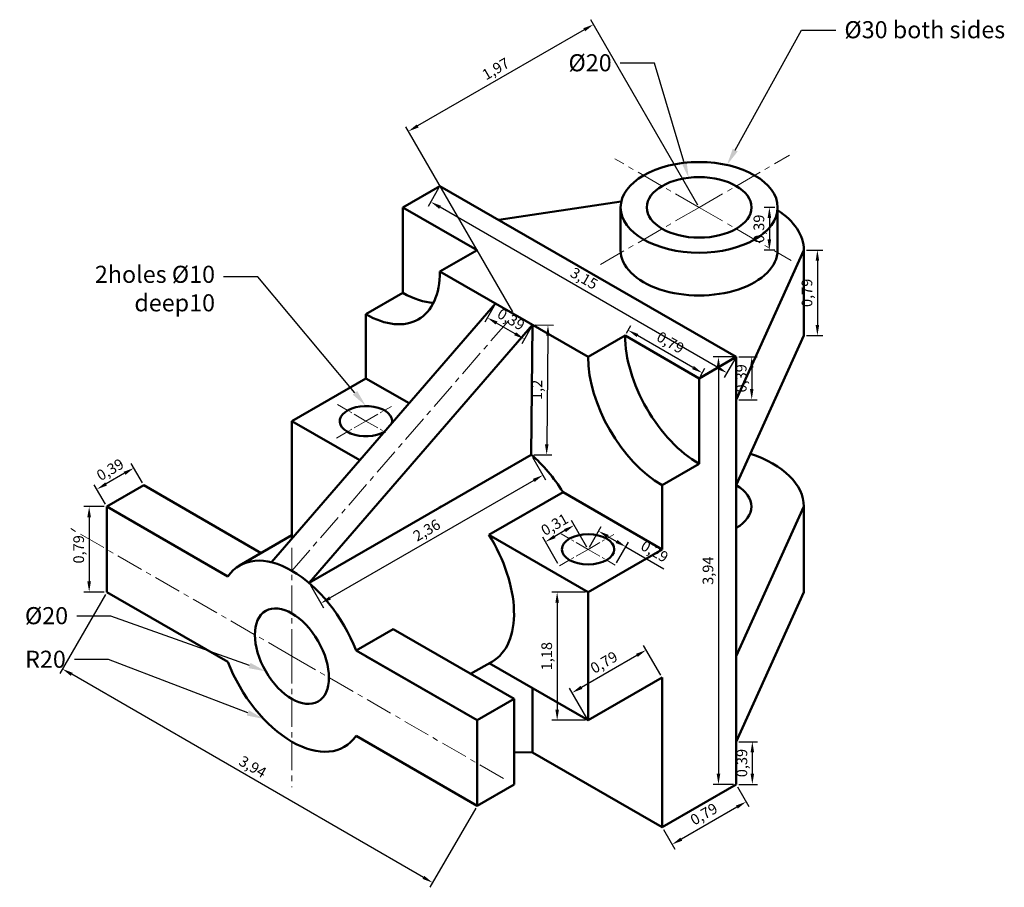
# Model space of a CAD drawing. Units: inches. Extents: x 1453 to 39065, y 1991 to 51453.
# Tile 1 of 1: x 1452.7 to 1683, y 1990.8 to 2193.8. Entities that reach past the tile are written whole.
import ezdxf
from ezdxf import colors
from ezdxf.entities.mleader import LeaderData, LeaderLine
from ezdxf.math import Vec2, Vec3

# ---------------------------------------------------------------- set-up
doc = ezdxf.new("R2010")
doc.units = ezdxf.units.IN
doc.linetypes.add('CENTER', pattern=[50.8, 31.75, -6.35, 6.35, -6.35])
for name, color, linetype, lineweight in [('M-CNTR', 1, 'CENTER', 18), ('M-DIMS', 2, 'Continuous', 25), ('M-OUTL', 7, 'Continuous', 50), ('M-TEXT', 3, 'Continuous', 25)]:
    doc.layers.add(name, color=color, linetype=linetype, lineweight=lineweight)
doc.styles.get("Standard").update_dxf_attribs({"font": 'arial.ttf'})
doc.dimstyles.new('ISO-25', dxfattribs={"dimtxt": 2.5, "dimasz": 2.5, "dimexe": 1.25, "dimexo": 0.625, "dimtad": 1, "dimtxsty": 'Standard', "dimcen": 2.5, "dimadec": 0, "dimazin": 0, "dimtfac": 1, "dimtmove": 0, "dimatfit": 3, "dimfxl": 1, "dimarcsym": 0})

# ---------------------------------------------------------------- blocks, each defined once
blk = doc.blocks.new('*D1')
at = {"layer": 'Defpoints', "color": 0, "transparency": 16777216}
for p in [(1563.98, 2127.35), (1562.07, 2124.04), (1572.64, 2122.35)]:
    blk.add_point(p, dxfattribs=at)
at = {"layer": 'M-DIMS', "color": 0, "lineweight": -2, "transparency": 16777216}
for p, q in [((1563.67, 2126.81), (1561.45, 2122.96)), ((1568.57, 2120.29), (1564.24, 2122.79)), ((1572.33, 2121.81), (1570.11, 2117.96))]:
    blk.add_line(p, q, dxfattribs=at)
at = {"layer": 'M-DIMS', "color": 0, "transparency": 16777216}
for points in [[(1564.45, 2123.15), (1564.03, 2122.43), (1562.07, 2124.04)], [(1568.78, 2120.65), (1568.36, 2119.93), (1570.73, 2119.04)]]:
    blk.add_solid(points, dxfattribs=at)
at = {"layer": 'M-DIMS', "color": 0, "transparency": 16777216, "insert": (1567.47, 2123.38), "char_height": 2.5, "attachment_point": 5, "rotation": 330}
blk.add_mtext('0,39', dxfattribs=at)
blk = doc.blocks.new('*D2')
at = {"layer": 'Defpoints', "color": 0, "transparency": 16777216}
for p in [(1543.6, 2167.65), (1611.62, 2149.85), (1568.31, 2124.85)]:
    blk.add_point(p, dxfattribs=at)
at = {"layer": 'M-DIMS', "color": 0, "lineweight": -2, "transparency": 16777216}
for p, q in [((1611.3, 2150.39), (1586.28, 2193.73)), ((1584.74, 2191.4), (1545.77, 2168.9)), ((1568, 2125.39), (1542.98, 2168.73))]:
    blk.add_line(p, q, dxfattribs=at)
at = {"layer": 'M-DIMS', "color": 0, "transparency": 16777216}
for points in [[(1584.53, 2191.76), (1584.95, 2191.04), (1586.91, 2192.65)], [(1545.56, 2169.26), (1545.98, 2168.54), (1543.6, 2167.65)]]:
    blk.add_solid(points, dxfattribs=at)
at = {"layer": 'M-DIMS', "color": 0, "transparency": 16777216, "insert": (1564.19, 2181.99), "char_height": 2.5, "attachment_point": 5, "rotation": 30}
blk.add_mtext('1,97', dxfattribs=at)
blk = doc.blocks.new('*D3')
at = {"layer": 'Defpoints', "color": 0, "transparency": 16777216}
for p in [(1550.99, 2154.85), (1548.85, 2151.13), (1620.28, 2114.85)]:
    blk.add_point(p, dxfattribs=at)
at = {"layer": 'M-DIMS', "color": 0, "lineweight": -2, "transparency": 16777216}
for p, q in [((1550.68, 2154.31), (1548.22, 2150.05)), ((1615.96, 2112.38), (1551.01, 2149.88)), ((1619.96, 2114.31), (1617.5, 2110.05))]:
    blk.add_line(p, q, dxfattribs=at)
at = {"layer": 'M-DIMS', "color": 0, "transparency": 16777216}
for points in [[(1551.22, 2150.24), (1550.8, 2149.52), (1548.85, 2151.13)], [(1616.17, 2112.74), (1615.75, 2112.02), (1618.13, 2111.13)]]:
    blk.add_solid(points, dxfattribs=at)
at = {"layer": 'M-DIMS', "color": 0, "transparency": 16777216, "insert": (1584.55, 2132.97), "char_height": 2.5, "attachment_point": 5, "rotation": 330}
blk.add_mtext('3,15', dxfattribs=at)
blk = doc.blocks.new('*D4')
at = {"layer": 'Defpoints', "color": 0, "transparency": 16777216}
for p in [(1629.99, 2149.85), (1628.05, 2139.85), (1629.99, 2139.85)]:
    blk.add_point(p, dxfattribs=at)
at = {"layer": 'M-DIMS', "color": 0, "lineweight": -2, "transparency": 16777216}
for p, q in [((1629.36, 2149.85), (1626.8, 2149.85)), ((1628.05, 2147.35), (1628.05, 2142.35)), ((1629.36, 2139.85), (1626.8, 2139.85))]:
    blk.add_line(p, q, dxfattribs=at)
at = {"layer": 'M-DIMS', "color": 0, "transparency": 16777216}
for points in [[(1627.63, 2147.35), (1628.47, 2147.35), (1628.05, 2149.85)], [(1627.63, 2142.35), (1628.47, 2142.35), (1628.05, 2139.85)]]:
    blk.add_solid(points, dxfattribs=at)
at = {"layer": 'M-DIMS', "color": 0, "transparency": 16777216, "insert": (1625.92, 2144.85), "char_height": 2.5, "attachment_point": 5, "rotation": 90}
blk.add_mtext('0,39', dxfattribs=at)
blk = doc.blocks.new('*D5')
at = {"layer": 'Defpoints', "color": 0, "transparency": 16777216}
for p in [(1620.28, 2114.85), (1620.28, 2104.85), (1623.92, 2104.85)]:
    blk.add_point(p, dxfattribs=at)
at = {"layer": 'M-DIMS', "color": 0, "lineweight": -2, "transparency": 16777216}
for p, q in [((1620.9, 2114.85), (1625.17, 2114.85)), ((1623.92, 2112.35), (1623.92, 2107.35)), ((1620.9, 2104.85), (1625.17, 2104.85))]:
    blk.add_line(p, q, dxfattribs=at)
at = {"layer": 'M-DIMS', "color": 0, "transparency": 16777216}
for points in [[(1623.5, 2112.35), (1624.34, 2112.35), (1623.92, 2114.85)], [(1623.5, 2107.35), (1624.34, 2107.35), (1623.92, 2104.85)]]:
    blk.add_solid(points, dxfattribs=at)
at = {"layer": 'M-DIMS', "color": 0, "transparency": 16777216, "insert": (1621.79, 2109.85), "char_height": 2.5, "attachment_point": 5, "rotation": 90}
blk.add_mtext('0,39', dxfattribs=at)
blk = doc.blocks.new('*D6')
at = {"layer": 'Defpoints', "color": 0, "transparency": 16777216}
for p in [(1636.11, 2139.85), (1636.11, 2119.85), (1639.28, 2119.85)]:
    blk.add_point(p, dxfattribs=at)
at = {"layer": 'M-DIMS', "color": 0, "lineweight": -2, "transparency": 16777216}
for p, q in [((1636.74, 2139.85), (1640.53, 2139.85)), ((1639.28, 2137.35), (1639.28, 2122.35)), ((1636.74, 2119.85), (1640.53, 2119.85))]:
    blk.add_line(p, q, dxfattribs=at)
at = {"layer": 'M-DIMS', "color": 0, "transparency": 16777216}
for points in [[(1638.87, 2137.35), (1639.7, 2137.35), (1639.28, 2139.85)], [(1638.87, 2122.35), (1639.7, 2122.35), (1639.28, 2119.85)]]:
    blk.add_solid(points, dxfattribs=at)
at = {"layer": 'M-DIMS', "color": 0, "transparency": 16777216, "insert": (1637.16, 2129.85), "char_height": 2.5, "attachment_point": 5, "rotation": 90}
blk.add_mtext('0,79', dxfattribs=at)
blk = doc.blocks.new('*D7')
at = {"layer": 'Defpoints', "color": 0, "transparency": 16777216}
for p in [(1620.28, 2114.85), (1616.14, 2014.85), (1620.28, 2014.85)]:
    blk.add_point(p, dxfattribs=at)
at = {"layer": 'M-DIMS', "color": 0, "lineweight": -2, "transparency": 16777216}
for p, q in [((1619.65, 2114.85), (1614.89, 2114.85)), ((1616.14, 2112.35), (1616.14, 2017.35)), ((1619.65, 2014.85), (1614.89, 2014.85))]:
    blk.add_line(p, q, dxfattribs=at)
at = {"layer": 'M-DIMS', "color": 0, "transparency": 16777216}
for points in [[(1615.72, 2112.35), (1616.56, 2112.35), (1616.14, 2114.85)], [(1615.72, 2017.35), (1616.56, 2017.35), (1616.14, 2014.85)]]:
    blk.add_solid(points, dxfattribs=at)
at = {"layer": 'M-DIMS', "color": 0, "transparency": 16777216, "insert": (1614.01, 2064.85), "char_height": 2.5, "attachment_point": 5, "rotation": 90}
blk.add_mtext('3,94', dxfattribs=at)
blk = doc.blocks.new('*D8')
at = {"layer": 'Defpoints', "color": 0, "transparency": 16777216}
for p in [(1620.28, 2024.85), (1620.28, 2014.85), (1624.06, 2014.85)]:
    blk.add_point(p, dxfattribs=at)
at = {"layer": 'M-DIMS', "color": 0, "lineweight": -2, "transparency": 16777216}
for p, q in [((1620.9, 2024.85), (1625.31, 2024.85)), ((1624.06, 2022.35), (1624.06, 2017.35)), ((1620.9, 2014.85), (1625.31, 2014.85))]:
    blk.add_line(p, q, dxfattribs=at)
at = {"layer": 'M-DIMS', "color": 0, "transparency": 16777216}
for points in [[(1623.65, 2022.35), (1624.48, 2022.35), (1624.06, 2024.85)], [(1623.65, 2017.35), (1624.48, 2017.35), (1624.06, 2014.85)]]:
    blk.add_solid(points, dxfattribs=at)
at = {"layer": 'M-DIMS', "color": 0, "transparency": 16777216, "insert": (1621.94, 2019.85), "char_height": 2.5, "attachment_point": 5, "rotation": 90}
blk.add_mtext('0,39', dxfattribs=at)
blk = doc.blocks.new('*D9')
at = {"layer": 'Defpoints', "color": 0, "transparency": 16777216}
for p in [(1473.05, 2079.85), (1468.92, 2059.85), (1473.05, 2059.85)]:
    blk.add_point(p, dxfattribs=at)
at = {"layer": 'M-DIMS', "color": 0, "lineweight": -2, "transparency": 16777216}
for p, q in [((1472.43, 2079.85), (1467.67, 2079.85)), ((1468.92, 2077.35), (1468.92, 2062.35)), ((1472.43, 2059.85), (1467.67, 2059.85))]:
    blk.add_line(p, q, dxfattribs=at)
at = {"layer": 'M-DIMS', "color": 0, "transparency": 16777216}
for points in [[(1468.5, 2077.35), (1469.34, 2077.35), (1468.92, 2079.85)], [(1468.5, 2062.35), (1469.34, 2062.35), (1468.92, 2059.85)]]:
    blk.add_solid(points, dxfattribs=at)
at = {"layer": 'M-DIMS', "color": 0, "transparency": 16777216, "insert": (1466.79, 2069.85), "char_height": 2.5, "attachment_point": 5, "rotation": 90}
blk.add_mtext('0,79', dxfattribs=at)
blk = doc.blocks.new('*D10')
at = {"layer": 'Defpoints', "color": 0, "transparency": 16777216}
for p in [(1620.28, 2014.85), (1602.96, 2004.85), (1605.29, 2000.8)]:
    blk.add_point(p, dxfattribs=at)
at = {"layer": 'M-DIMS', "color": 0, "lineweight": -2, "transparency": 16777216}
for p, q in [((1620.59, 2014.31), (1623.24, 2009.72)), ((1620.45, 2009.55), (1607.46, 2002.05)), ((1603.27, 2004.31), (1605.92, 1999.72))]:
    blk.add_line(p, q, dxfattribs=at)
at = {"layer": 'M-DIMS', "color": 0, "transparency": 16777216}
for points in [[(1620.24, 2009.91), (1620.66, 2009.19), (1622.61, 2010.8)], [(1607.25, 2002.41), (1607.67, 2001.69), (1605.29, 2000.8)]]:
    blk.add_solid(points, dxfattribs=at)
at = {"layer": 'M-DIMS', "color": 0, "transparency": 16777216, "insert": (1612.89, 2007.64), "char_height": 2.5, "attachment_point": 5, "rotation": 30}
blk.add_mtext('0,79', dxfattribs=at)
blk = doc.blocks.new('*D11')
at = {"layer": 'Defpoints', "color": 0, "transparency": 16777216}
for p in [(1473.05, 2059.85), (1462.67, 2041.86), (1559.65, 2009.85)]:
    blk.add_point(p, dxfattribs=at)
at = {"layer": 'M-DIMS', "color": 0, "lineweight": -2, "transparency": 16777216}
for p, q in [((1472.74, 2059.31), (1462.04, 2040.78)), ((1547.11, 1993.11), (1464.83, 2040.61)), ((1559.34, 2009.31), (1548.65, 1990.78))]:
    blk.add_line(p, q, dxfattribs=at)
at = {"layer": 'M-DIMS', "color": 0, "transparency": 16777216}
for points in [[(1465.04, 2040.97), (1464.62, 2040.25), (1462.67, 2041.86)], [(1547.31, 1993.47), (1546.9, 1992.75), (1549.27, 1991.86)]]:
    blk.add_solid(points, dxfattribs=at)
at = {"layer": 'M-DIMS', "color": 0, "transparency": 16777216, "insert": (1507.03, 2018.71), "char_height": 2.5, "attachment_point": 5, "rotation": 330}
blk.add_mtext('3,94', dxfattribs=at)
blk = doc.blocks.new('*D12')
at = {"layer": 'Defpoints', "color": 0, "transparency": 16777216}
for p in [(1602.96, 2039.85), (1581.91, 2036.3), (1585.63, 2029.85)]:
    blk.add_point(p, dxfattribs=at)
at = {"layer": 'M-DIMS', "color": 0, "lineweight": -2, "transparency": 16777216}
for p, q in [((1602.64, 2040.39), (1598.61, 2047.38)), ((1597.07, 2045.05), (1584.08, 2037.55)), ((1585.32, 2030.39), (1581.29, 2037.38))]:
    blk.add_line(p, q, dxfattribs=at)
at = {"layer": 'M-DIMS', "color": 0, "transparency": 16777216}
for points in [[(1596.86, 2045.41), (1597.27, 2044.69), (1599.23, 2046.3)], [(1583.87, 2037.91), (1584.28, 2037.19), (1581.91, 2036.3)]]:
    blk.add_solid(points, dxfattribs=at)
at = {"layer": 'M-DIMS', "color": 0, "transparency": 16777216, "insert": (1589.51, 2043.14), "char_height": 2.5, "attachment_point": 5, "rotation": 30}
blk.add_mtext('0,79', dxfattribs=at)
blk = doc.blocks.new('*D13')
at = {"layer": 'Defpoints', "color": 0, "transparency": 16777216}
for p in [(1585.63, 2059.85), (1578.4, 2029.85), (1585.63, 2029.85)]:
    blk.add_point(p, dxfattribs=at)
at = {"layer": 'M-DIMS', "color": 0, "lineweight": -2, "transparency": 16777216}
for p, q in [((1585.01, 2059.85), (1577.15, 2059.85)), ((1578.4, 2057.35), (1578.4, 2032.35)), ((1585.01, 2029.85), (1577.15, 2029.85))]:
    blk.add_line(p, q, dxfattribs=at)
at = {"layer": 'M-DIMS', "color": 0, "transparency": 16777216}
for points in [[(1577.99, 2057.35), (1578.82, 2057.35), (1578.4, 2059.85)], [(1577.99, 2032.35), (1578.82, 2032.35), (1578.4, 2029.85)]]:
    blk.add_solid(points, dxfattribs=at)
at = {"layer": 'M-DIMS', "color": 0, "transparency": 16777216, "insert": (1576.28, 2044.85), "char_height": 2.5, "attachment_point": 5, "rotation": 90}
blk.add_mtext('1,18', dxfattribs=at)
blk = doc.blocks.new('*D14')
at = {"layer": 'Defpoints', "color": 0, "transparency": 16777216}
for p in [(1575.66, 2071.6), (1585.63, 2069.85), (1578.91, 2065.97)]:
    blk.add_point(p, dxfattribs=at)
at = {"layer": 'M-DIMS', "color": 0, "lineweight": -2, "transparency": 16777216}
for p, q in [((1585.32, 2070.39), (1581.76, 2076.56)), ((1580.22, 2074.23), (1577.83, 2072.85)), ((1578.6, 2066.51), (1575.04, 2072.68))]:
    blk.add_line(p, q, dxfattribs=at)
at = {"layer": 'M-DIMS', "color": 0, "transparency": 16777216}
for points in [[(1580.01, 2074.59), (1580.43, 2073.87), (1582.38, 2075.48)], [(1577.62, 2073.21), (1578.04, 2072.49), (1575.66, 2071.6)]]:
    blk.add_solid(points, dxfattribs=at)
at = {"layer": 'M-DIMS', "color": 0, "transparency": 16777216, "insert": (1577.96, 2075.38), "char_height": 2.5, "attachment_point": 5, "rotation": 30}
blk.add_mtext('0,31', dxfattribs=at)
blk = doc.blocks.new('*D15')
at = {"layer": 'Defpoints', "color": 0, "transparency": 16777216}
for p in [(1585.63, 2069.85), (1594.45, 2070.45), (1591.99, 2066.18)]:
    blk.add_point(p, dxfattribs=at)
at = {"layer": 'M-DIMS', "color": 0, "lineweight": -2, "transparency": 16777216}
for p, q in [((1585.95, 2070.39), (1588.72, 2075.2)), ((1590.26, 2072.86), (1592.29, 2071.7)), ((1592.3, 2066.72), (1595.08, 2071.53)), ((1594.45, 2070.45), (1603.33, 2065.32))]:
    blk.add_line(p, q, dxfattribs=at)
at = {"layer": 'M-DIMS', "color": 0, "transparency": 16777216}
for points in [[(1590.47, 2073.22), (1590.05, 2072.5), (1588.1, 2074.11)], [(1592.5, 2072.06), (1592.08, 2071.33), (1594.45, 2070.45)]]:
    blk.add_solid(points, dxfattribs=at)
at = {"layer": 'M-DIMS', "color": 0, "transparency": 16777216, "insert": (1601.04, 2069.1), "char_height": 2.5, "attachment_point": 5, "rotation": 330}
blk.add_mtext('0,29', dxfattribs=at)
blk = doc.blocks.new('*D16')
at = {"layer": 'Defpoints', "color": 0, "transparency": 16777216}
for p in [(1594.3, 2119.85), (1595.03, 2121.12), (1611.62, 2109.85)]:
    blk.add_point(p, dxfattribs=at)
at = {"layer": 'M-DIMS', "color": 0, "lineweight": -2, "transparency": 16777216}
for p, q in [((1594.61, 2120.39), (1595.65, 2122.2)), ((1610.18, 2112.37), (1597.19, 2119.87)), ((1611.93, 2110.39), (1612.97, 2112.2))]:
    blk.add_line(p, q, dxfattribs=at)
at = {"layer": 'M-DIMS', "color": 0, "transparency": 16777216}
for points in [[(1597.4, 2120.23), (1596.99, 2119.51), (1595.03, 2121.12)], [(1610.39, 2112.73), (1609.98, 2112.01), (1612.35, 2111.12)]]:
    blk.add_solid(points, dxfattribs=at)
at = {"layer": 'M-DIMS', "color": 0, "transparency": 16777216, "insert": (1604.75, 2117.96), "char_height": 2.5, "attachment_point": 5, "rotation": 330}
blk.add_mtext('0,79', dxfattribs=at)
blk = doc.blocks.new('*D17')
at = {"layer": 'Defpoints', "color": 0, "transparency": 16777216}
for p in [(1572.33, 2091.98), (1520.37, 2061.98), (1523.12, 2057.22)]:
    blk.add_point(p, dxfattribs=at)
at = {"layer": 'M-DIMS', "color": 0, "lineweight": -2, "transparency": 16777216}
for p, q in [((1572.64, 2091.44), (1575.71, 2086.13)), ((1572.92, 2085.97), (1525.29, 2058.47)), ((1520.68, 2061.44), (1523.75, 2056.13))]:
    blk.add_line(p, q, dxfattribs=at)
at = {"layer": 'M-DIMS', "color": 0, "transparency": 16777216}
for points in [[(1572.71, 2086.33), (1573.13, 2085.61), (1575.08, 2087.22)], [(1525.08, 2058.83), (1525.49, 2058.11), (1523.12, 2057.22)]]:
    blk.add_solid(points, dxfattribs=at)
at = {"layer": 'M-DIMS', "color": 0, "transparency": 16777216, "insert": (1548.04, 2074.06), "char_height": 2.5, "attachment_point": 5, "rotation": 30}
blk.add_mtext('2,36', dxfattribs=at)
blk = doc.blocks.new('*D18')
at = {"layer": 'Defpoints', "color": 0, "transparency": 16777216}
for p in [(1572.64, 2122.35), (1572.33, 2091.98), (1575.94, 2091.95)]:
    blk.add_point(p, dxfattribs=at)
at = {"layer": 'M-DIMS', "color": 0, "lineweight": -2, "transparency": 16777216}
for p, q in [((1573.27, 2122.34), (1577.51, 2122.3)), ((1576.23, 2119.81), (1575.97, 2094.45)), ((1572.95, 2091.98), (1577.19, 2091.93))]:
    blk.add_line(p, q, dxfattribs=at)
at = {"layer": 'M-DIMS', "color": 0, "transparency": 16777216}
for points in [[(1575.82, 2119.81), (1576.65, 2119.81), (1576.26, 2122.31)], [(1575.55, 2094.45), (1576.39, 2094.44), (1575.94, 2091.95)]]:
    blk.add_solid(points, dxfattribs=at)
at = {"layer": 'M-DIMS', "color": 0, "transparency": 16777216, "insert": (1573.97, 2107.15), "char_height": 2.5, "attachment_point": 5, "rotation": 89.4064}
blk.add_mtext('1,2', dxfattribs=at)
blk = doc.blocks.new('*D19')
at = {"layer": 'Defpoints', "color": 0, "transparency": 16777216}
for p in [(1481.71, 2084.85), (1470.72, 2083.89), (1473.05, 2079.85)]:
    blk.add_point(p, dxfattribs=at)
at = {"layer": 'M-DIMS', "color": 0, "lineweight": -2, "transparency": 16777216}
for p, q in [((1481.4, 2085.39), (1478.75, 2089.97)), ((1477.21, 2087.64), (1472.88, 2085.14)), ((1472.74, 2080.39), (1470.09, 2084.97))]:
    blk.add_line(p, q, dxfattribs=at)
at = {"layer": 'M-DIMS', "color": 0, "transparency": 16777216}
for points in [[(1477.01, 2088), (1477.42, 2087.28), (1479.38, 2088.89)], [(1472.68, 2085.5), (1473.09, 2084.78), (1470.72, 2083.89)]]:
    blk.add_solid(points, dxfattribs=at)
at = {"layer": 'M-DIMS', "color": 0, "transparency": 16777216, "insert": (1473.99, 2088.23), "char_height": 2.5, "attachment_point": 5, "rotation": 30}
blk.add_mtext('0,39', dxfattribs=at)

msp = doc.modelspace()

# ---------------------------------------------------------------- linework, layer by layer
at = {"layer": 'M-CNTR', "ltscale": 0.2}
for p, q in [((1611.616, 2149.848), (1591.894, 2161.234)), ((1611.616, 2149.848), (1632.787, 2162.071)), ((1611.616, 2149.848), (1588.044, 2136.239)), ((1611.616, 2149.848), (1633.15, 2137.415)), ((1516.353, 2064.848), (1568.314, 2124.848)), ((1516.353, 2044.848), (1463.962, 2075.095)), ((1516.353, 2044.848), (1516.353, 2070.202)), ((1516.353, 2044.848), (1516.353, 2014.177)), ((1516.353, 2044.848), (1566.878, 2015.677))]:
    msp.add_line(p, q, dxfattribs=at)
at = {"layer": 'M-CNTR', "ltscale": 0.1}
for p, q in [((1533.673, 2099.848), (1526.996, 2103.703)), ((1533.673, 2099.848), (1539.626, 2103.284)), ((1533.673, 2099.848), (1526.754, 2095.853)), ((1533.673, 2099.848), (1538.226, 2097.219)), ((1585.635, 2069.848), (1579.354, 2073.474)), ((1585.635, 2069.848), (1591.675, 2073.335)), ((1585.635, 2069.848), (1578.914, 2065.967)), ((1585.635, 2069.848), (1591.99, 2066.179))]:
    msp.add_line(p, q, dxfattribs=at)
at = {"layer": 'M-OUTL'}
for p, q in [((1550.994, 2154.848), (1542.334, 2149.848)), ((1620.276, 2114.848), (1550.994, 2154.848)), ((1542.334, 2149.848), (1559.654, 2139.848)), ((1542.334, 2149.848), (1542.334, 2129.848)), ((1564.727, 2146.919), (1593.404, 2151.244)), ((1593.244, 2149.848), (1593.244, 2139.848)), ((1629.987, 2149.848), (1629.987, 2139.848)), ((1559.654, 2139.848), (1550.994, 2134.848)), ((1620.276, 2104.848), (1636.11, 2139.848)), ((1636.11, 2139.848), (1636.11, 2119.848)), ((1550.994, 2134.848), (1585.635, 2114.848)), ((1542.334, 2129.848), (1533.673, 2124.848)), ((1511.575, 2066.83), (1563.984, 2127.348)), ((1533.673, 2109.848), (1533.673, 2124.848)), ((1520.368, 2061.985), (1572.644, 2122.348)), ((1572.33, 2091.985), (1572.644, 2122.348)), ((1594.295, 2119.848), (1585.635, 2114.848)), ((1611.616, 2109.848), (1594.295, 2119.848)), ((1620.276, 2084.848), (1636.11, 2119.848)), ((1620.276, 2114.848), (1611.616, 2109.848)), ((1620.276, 2014.848), (1620.276, 2114.848)), ((1620.276, 2114.848), (1620.276, 2104.848)), ((1516.353, 2099.848), (1533.673, 2109.848)), ((1543.777, 2104.015), (1533.673, 2109.848)), ((1611.616, 2109.848), (1611.616, 2089.848)), ((1516.353, 2099.848), (1516.353, 2072.348)), ((1532.23, 2090.681), (1516.353, 2099.848)), ((1520.368, 2061.985), (1572.33, 2091.985)), ((1611.616, 2089.848), (1602.955, 2084.848)), ((1473.052, 2079.848), (1481.712, 2084.848)), ((1481.712, 2084.848), (1509.178, 2068.99)), ((1602.955, 2084.848), (1602.955, 2069.848)), ((1562.45, 2073.233), (1579.771, 2083.233)), ((1602.955, 2069.848), (1579.771, 2083.233)), ((1473.052, 2069.848), (1473.052, 2079.848)), ((1473.052, 2079.848), (1501.353, 2063.508)), ((1550.994, 2079.848), (1550.994, 2079.666)), ((1551.151, 2079.757), (1550.994, 2079.848)), ((1620.276, 2044.848), (1636.11, 2079.848)), ((1636.11, 2079.848), (1636.11, 2059.848)), ((1504.105, 2066.061), (1516.353, 2073.132)), ((1585.635, 2059.848), (1562.45, 2073.233)), ((1473.052, 2069.848), (1473.052, 2059.848)), ((1602.955, 2069.848), (1585.635, 2059.848)), ((1473.052, 2059.848), (1501.353, 2043.508)), ((1585.635, 2059.848), (1585.635, 2029.848)), ((1620.276, 2024.848), (1636.11, 2059.848)), ((1531.353, 2046.188), (1540.013, 2051.188)), ((1568.314, 2034.848), (1540.013, 2051.188)), ((1559.654, 2029.848), (1531.353, 2046.188)), ((1559.654, 2029.848), (1533.673, 2044.848)), ((1558.168, 2040.706), (1563.241, 2043.635)), ((1585.635, 2029.848), (1562.498, 2043.206)), ((1585.635, 2029.848), (1602.955, 2039.848)), ((1602.955, 2039.848), (1602.955, 2004.848)), ((1572.644, 2022.348), (1572.644, 2037.348)), ((1559.654, 2029.848), (1568.314, 2034.848)), ((1568.314, 2034.848), (1568.314, 2014.848)), ((1559.654, 2019.848), (1559.654, 2029.848)), ((1559.654, 2009.848), (1531.353, 2026.188)), ((1568.314, 2022.408), (1572.644, 2022.348)), ((1602.955, 2004.848), (1572.644, 2022.348)), ((1559.654, 2019.848), (1559.654, 2009.848)), ((1568.314, 2014.848), (1559.654, 2009.848)), ((1602.955, 2004.848), (1620.276, 2014.848))]:
    msp.add_line(p, q, dxfattribs=at)
for centre, major_axis in [((1611.616, 2149.848), (-18.371, 0)), ((1611.616, 2149.848), (-12.247, 0)), ((1585.635, 2069.848), (-6.124, 0)), ((1516.353, 2044.848), (6.124, -10.607))]:
    msp.add_ellipse(centre, major_axis=major_axis, ratio=0.5773503, dxfattribs=at)
for centre, major_axis, start_param, end_param in [((1611.616, 2139.848), (-24.495, 0), 5.558483, 5.5604511), ((1611.616, 2139.848), (-24.495, 0), 3.1415927, 3.866295), ((1611.616, 2139.848), (-18.371, 0), 0, 3.1415927), ((1533.673, 2144.848), (12.247, -21.213), 5.4977871, 7.0685835), ((1542.334, 2149.848), (12.247, -21.213), 5.4977871, 5.9218182), ((1611.616, 2109.848), (12.247, -21.213), 10.2101761, 11.7809725), ((1602.955, 2104.848), (12.247, -21.213), 3.9269908, 5.4977871), ((1533.673, 2099.848), (-6.124, 0), 2.9996956, 8.6393798), ((1568.314, 2074.848), (12.247, -21.213), 1.6334602, 2.1222293), ((1611.616, 2079.848), (-24.495, 0), 3.1415927, 4.2013982), ((1611.616, 2079.848), (-12.247, 0), 8.6393798, 10.2101761), ((1550.994, 2064.848), (12.247, -21.213), 6.2831853, 7.9166455), ((1516.353, 2044.848), (12.247, -21.213), 1.3089969, 3.403392), ((1516.353, 2044.848), (12.247, -21.213), 4.4505896, 6.5449847)]:
    msp.add_ellipse(centre, major_axis=major_axis, ratio=0.5773503, start_param=start_param, end_param=end_param, dxfattribs=at)

# ---------------------------------------------------------------- dimensions: what is measured, and where the dimension line sits
at = {"layer": 'M-DIMS'}
for base, p1, p2, angle, picture, middle in [((1543.605, 2167.646), (1611.616, 2149.848), (1568.314, 2124.848), 210, '*D2', (1564.192, 2181.989)), ((1548.846, 2151.128), (1620.276, 2114.848), (1550.994, 2154.848), 150, '*D3', (1584.551, 2132.97)), ((1628.049, 2139.848), (1629.987, 2149.848), (1629.987, 2139.848), 270, '*D4', (1625.922, 2144.848)), ((1639.284, 2119.848), (1636.11, 2139.848), (1636.11, 2119.848), 270, '*D6', (1637.156, 2129.848)), ((1562.074, 2124.039), (1572.644, 2122.348), (1563.984, 2127.348), 150, '*D1', (1567.468, 2123.381)), ((1575.944, 2091.947), (1572.644, 2122.348), (1572.33, 2091.985), 269.40637, '*D18', (1573.974, 2107.151)), ((1595.029, 2121.118), (1611.616, 2109.848), (1594.295, 2119.848), 150, '*D16', (1604.753, 2117.961)), ((1616.141, 2014.848), (1620.276, 2114.848), (1620.276, 2014.848), 270, '*D7', (1614.014, 2064.848)), ((1623.919, 2104.848), (1620.276, 2114.848), (1620.276, 2104.848), 270, '*D5', (1621.791, 2109.848)), ((1470.719, 2083.888), (1481.712, 2084.848), (1473.052, 2079.848), 210, '*D19', (1473.985, 2088.23)), ((1523.121, 2057.217), (1572.33, 2091.985), (1520.368, 2061.985), 210, '*D17', (1548.038, 2074.059)), ((1468.92, 2059.848), (1473.052, 2079.848), (1473.052, 2059.848), 270, '*D9', (1466.792, 2069.848)), ((1575.664, 2071.597), (1585.635, 2069.848), (1578.914, 2065.967), 210, '*D14', (1577.961, 2075.379)), ((1594.453, 2070.445), (1585.635, 2069.848), (1591.99, 2066.179), 330, '*D15', (1601.037, 2069.1)), ((1462.668, 2041.863), (1559.654, 2009.848), (1473.052, 2059.848), 150, '*D11', (1507.033, 2018.705)), ((1578.405, 2029.848), (1585.635, 2059.848), (1585.635, 2029.848), 270, '*D13', (1576.278, 2044.848)), ((1581.911, 2036.298), (1602.955, 2039.848), (1585.635, 2029.848), 210, '*D12', (1589.507, 2043.14)), ((1624.064, 2014.848), (1620.276, 2024.848), (1620.276, 2014.848), 270, '*D8', (1621.936, 2019.848)), ((1605.294, 2000.798), (1620.276, 2014.848), (1602.955, 2004.848), 210, '*D10', (1612.89, 2007.64))]:
    dim = msp.add_linear_dim(base=base, p1=p1, p2=p2, angle=angle, dimstyle='ISO-25', override={"dimlfac": 0.03937, "dimrnd": 0}, dxfattribs=at)
    dim.commit()
    dim.dimension.update_dxf_attribs({"geometry": picture, "text_midpoint": middle})

# ---------------------------------------------------------------- leaders
at = {"layer": 'M-TEXT'}
ml = msp.add_multileader_mtext('Standard', dxfattribs=at)
ml.set_content('%%C30 both sides', color=256)
ml.set_leader_properties()
ml.build(insert=Vec2(0, 0))
ctx = ml.context
ctx.base_point, ctx.plane_origin = Vec3(1643.596, 2191.337), Vec3(1618.126, 2159.766)
notes = []
notes.append((ctx, [(0, (1, 1, 0), (1635.596, 2191.337), (1, 0), 8, [(0, [(1618.126, 2159.766)], 0, [])])]))
ctx.mtext.insert, ctx.mtext.flow_direction = Vec3(1645.596, 2193.418), 5
ml = msp.add_multileader_mtext('Standard', dxfattribs=at)
ml.set_content('%%C20', color=256)
ml.set_leader_properties()
ml.build(insert=Vec2(0, 0))
ctx = ml.context
ctx.base_point, ctx.plane_origin = Vec3(1579.09, 2183.608), Vec3(1609.173, 2156.777)
ctx.text_align_type = 2
notes.append((ctx, [(0, (1, 1, 0), (1601.158, 2183.608), (-1, 0), 8, [(0, [(1609.173, 2156.777)], 0, [])])]))
ctx.mtext.insert, ctx.mtext.alignment, ctx.mtext.flow_direction = Vec3(1591.158, 2185.689), 3, 5
ml = msp.add_multileader_mtext('Standard', dxfattribs=at)
ml.set_content('2holes %%C10 \\Pdeep10', color=256)
ml.set_leader_properties()
ml.build(insert=Vec2(0, 0))
ctx = ml.context
ctx.base_point, ctx.plane_origin = Vec3(1468.213, 2133.636), Vec3(1533.673, 2103.383)
ctx.text_align_type = 2
notes.append((ctx, [(0, (1, 1, 0), (1508.363, 2133.636), (-1, 0), 8, [(0, [(1533.673, 2103.383)], 0, [])])]))
ctx.mtext.insert, ctx.mtext.alignment, ctx.mtext.flow_direction = Vec3(1498.363, 2136.191), 3, 5
ml = msp.add_multileader_mtext('Standard', dxfattribs=at)
ml.set_content('%%C20', color=256)
ml.set_leader_properties()
ml.build(insert=Vec2(0, 0))
ctx = ml.context
ctx.base_point, ctx.plane_origin = Vec3(1451.931, 2054.251), Vec3(1510.229, 2041.312)
ctx.text_align_type = 2
notes.append((ctx, [(0, (1, 1, 0), (1473.999, 2054.251), (-1, 0), 8, [(0, [(1510.229, 2041.312)], 0, [])])]))
ctx.mtext.insert, ctx.mtext.alignment, ctx.mtext.flow_direction = Vec3(1463.999, 2056.331), 3, 5
ml = msp.add_multileader_mtext('Standard', dxfattribs=at)
ml.set_content('R20', color=256)
ml.set_leader_properties()
ml.build(insert=Vec2(0, 0))
ctx = ml.context
ctx.base_point, ctx.plane_origin = Vec3(1451.919, 2044.101), Vec3(1509.761, 2030.159)
ctx.text_align_type = 2
notes.append((ctx, [(0, (1, 1, 0), (1473.463, 2044.101), (-1, 0), 8, [(0, [(1509.761, 2030.159)], 0, [])])]))
ctx.mtext.insert, ctx.mtext.alignment, ctx.mtext.flow_direction = Vec3(1463.463, 2046.135), 3, 5
for ctx, leaders in notes:
    for number, flags, end, landing, length, lines in leaders:
        leader = LeaderData()
        leader.index, (leader.has_last_leader_line, leader.has_dogleg_vector, leader.attachment_direction) = number, flags
        leader.last_leader_point, leader.dogleg_vector, leader.dogleg_length = Vec3(end), Vec3(landing), length
        for number, points, colour, breaks in lines:
            line = LeaderLine()
            line.index, line.vertices, line.color, line.breaks = number, Vec3.list(points), colors.encode_raw_color(colour), breaks
            leader.lines.append(line)
        ctx.leaders.append(leader)

doc.saveas('drawing.dxf')
